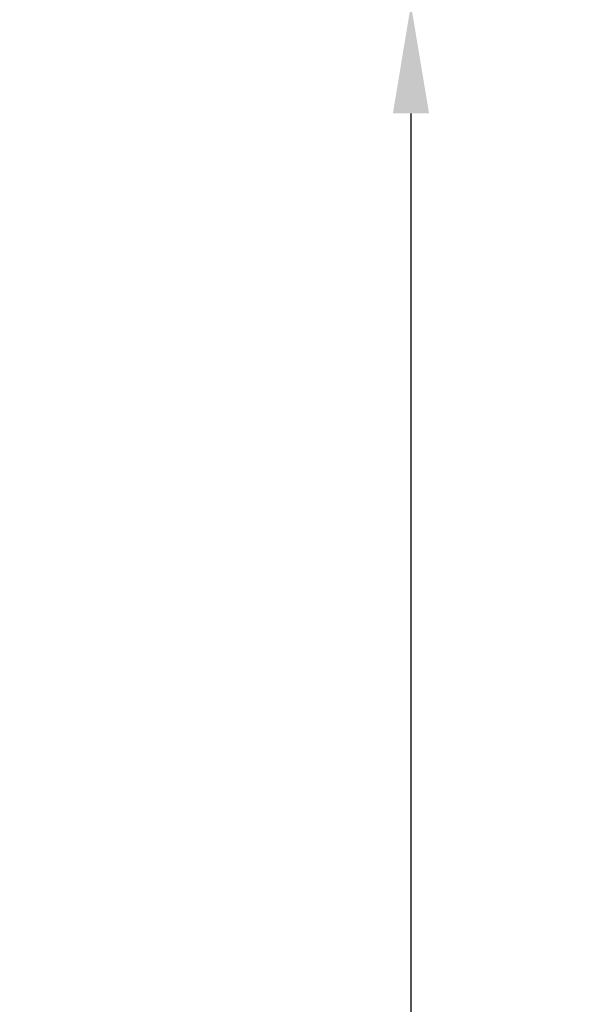
# Model space of a CAD drawing. Units: inches. Extents: x -301 to 715, y -607 to 364.
# Tile 113 of 141: x 16 to 42, y 147 to 192. Entities that reach past the tile are written whole.
import ezdxf

# ---------------------------------------------------------------- set-up
doc = ezdxf.new("R2010")
doc.units = ezdxf.units.IN
doc.header["$MEASUREMENT"] = 0
doc.layers.add('A-ANNO-DIMS', color=2, linetype='Continuous', lineweight=18)
doc.styles.get("Standard").update_dxf_attribs({"font": 'arial.ttf'})
doc.dimstyles.get("Standard").update_dxf_attribs({"dimtxt": 0.18, "dimasz": 0.18, "dimexe": 0.18, "dimexo": 0.0625, "dimgap": 0.09, "dimtad": 0, "dimtih": 1, "dimtoh": 1, "dimdec": 1, "dimzin": 0, "dimdsep": 46, "dimlunit": 4, "dimtxsty": 'Standard', "dimcen": 0.09, "dimclrd": 3, "dimclre": 4, "dimclrt": 6, "dimadec": 0, "dimazin": 0, "dimtfac": 1, "dimtdec": 1, "dimtofl": 0, "dimtmove": 0, "dimatfit": 3, "dimfxl": 1, "dimtfill": 2, "dimtfillclr": 51, "dimtolj": 1, "dimtzin": 0, "dimarcsym": 0})

# ---------------------------------------------------------------- blocks, each defined once
blk = doc.blocks.new('*D49')
at = {"layer": 'A-ANNO-DIMS', "color": 0, "lineweight": -2, "transparency": 16777216}
for p, q in [((15.959, 193.182), (34.084, 193.182)), ((33.904, 188.182), (33.904, 93.304)), ((33.904, -4.818), (33.904, 90.061)), ((21.959, -9.818), (34.084, -9.818))]:
    blk.add_line(p, q, dxfattribs=at)
at = {"layer": 'A-ANNO-DIMS', "color": 0, "transparency": 16777216}
for points in [[(33.071, 188.182), (34.737, 188.182), (33.904, 193.182)], [(33.071, -4.818), (34.737, -4.818), (33.904, -9.818)]]:
    blk.add_solid(points, dxfattribs=at)
at = {"layer": 'Defpoints', "color": 0, "transparency": 16777216}
for p in [(15.897, 193.182), (33.904, 193.182), (21.897, -9.818)]:
    blk.add_point(p, dxfattribs=at)
at = {"layer": 'A-ANNO-DIMS', "color": 0, "transparency": 16777216, "insert": (33.904, 91.682), "char_height": 3, "attachment_point": 5, "bg_fill": 1, "box_fill_scale": 1.25, "bg_fill_color": 51, "bg_fill_transparency": 0}
blk.add_mtext('\\A1;16\'-11"', dxfattribs=at)

msp = doc.modelspace()

# ---------------------------------------------------------------- dimensions: what is measured, and where the dimension line sits
at = {"layer": 'A-ANNO-DIMS'}
dim = msp.add_linear_dim(base=(33.904, 193.182), p1=(21.897, -9.818), p2=(15.897, 193.182), angle=90, dimstyle='Standard', override={"dimtxt": 3, "dimasz": 5, "dimclrd": 0, "dimclre": 0, "dimclrt": 0}, dxfattribs=at)
dim.commit()
dim.dimension.update_dxf_attribs({"geometry": '*D49', "text_midpoint": (33.904, 91.682)})

doc.saveas('drawing.dxf')
